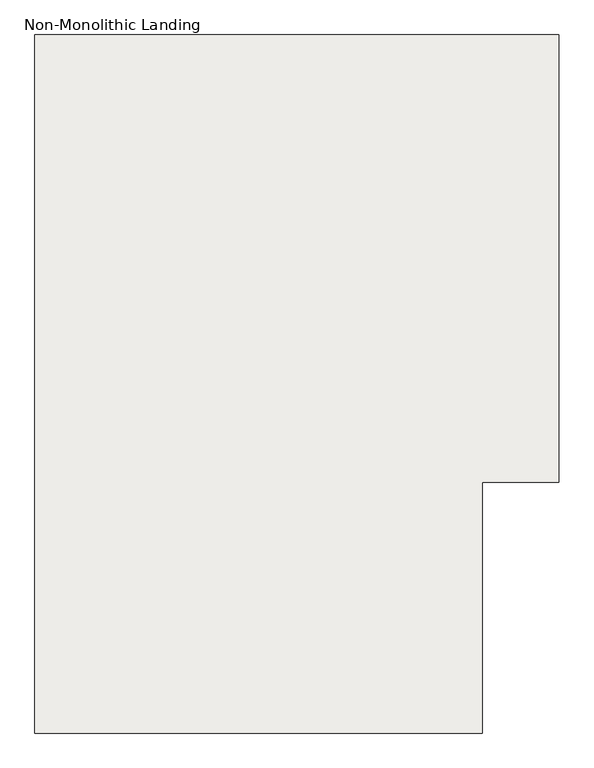
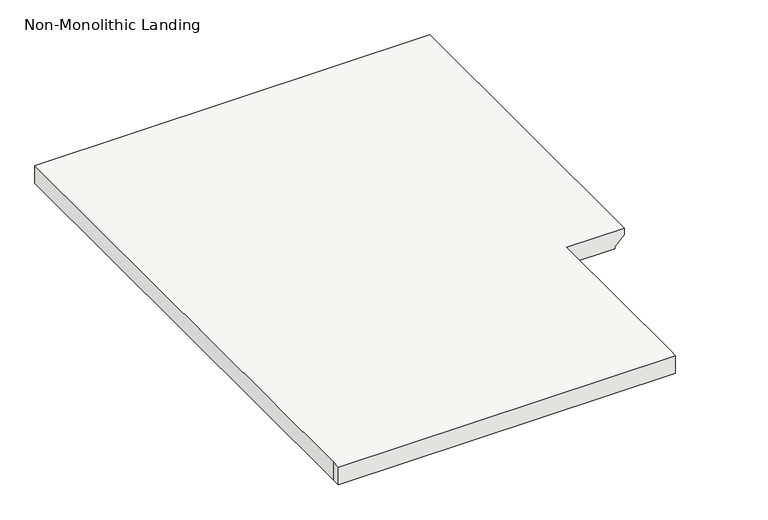
"""IFC4 building model written with IfcOpenShell, lengths in millimetres: slab geometry, Non-Monolithic Landing."""

from ifc_helpers import new_model, si_unit, origin, place, context, project, spatial, faceted_brep, source, transform, mapped, element, save


def non_monolithic_landing_bb2b3a88(model_context):
    return source(origin(), model_context, "Body", "Brep", [
        faceted_brep([(-10197.3156858, 1045.1115003, 1132.4166667), (-10197.3156858, 1045.1115003, 1151.4666667), (-10197.3156858, 130.7115003, 1151.4666667), (-10197.3156858, 130.7115003, 1132.4166667), (-10222.7156858, 1045.1115003, 1107.0166667), (-10222.7156858, 130.7115003, 1107.0166667), (-11268.1522729, 1045.1115003, 1151.4666667), (-11268.1522729, -356.3993654, 1151.4666667), (-11268.1522729, -381.7993654, 1151.4666667), (-10353.7522729, -381.7993654, 1151.4666667), (-10353.7522729, -356.3993654, 1151.4666667), (-10353.7522729, 130.7115003, 1151.4666667), (-10222.7156858, 1045.1115003, 1100.6666667), (-10222.7156858, 130.7115003, 1100.6666667), (-10353.7522729, 130.7115003, 1100.6666667), (-10353.7522729, -356.3993654, 1100.6666667), (-10353.7522729, -381.7993654, 1100.6666667), (-11268.1522729, -381.7993654, 1100.6666667), (-11268.1522729, -356.3993654, 1100.6666667), (-11268.1522729, 1045.1115003, 1100.6666667)], [[[0, 1, 2, 3]], [[4, 0, 3, 5]], [[6, 7, 8, 9, 10, 11, 2, 1]], [[12, 13, 14, 15, 16, 17, 18, 19]], [[13, 12, 4, 5]], [[6, 1, 0, 4, 12, 19]], [[7, 6, 19, 18]], [[8, 7, 18, 17]], [[9, 8, 17, 16]], [[10, 9, 16, 15]], [[11, 10, 15, 14]], [[2, 11, 14, 13, 5, 3]]]),
    ])


if __name__ == "__main__":
    model = new_model("IFC4")
    model_context = context("Model", 3, world=origin())
    ifc_project = project(units=[si_unit("LENGTHUNIT", "METRE", prefix="MILLI")], contexts=[model_context])
    site = spatial("IfcSite", under=ifc_project)
    building = spatial("IfcBuilding", under=site)
    placement = place(None, origin())
    non_monolithic_landing_shape = non_monolithic_landing_bb2b3a88(model_context)
    element("IfcSlab", 1, ObjectType="Non-Monolithic Landing", at=placement, inside=building, context=model_context, shape_type="MappedRepresentation", body=[
        mapped(non_monolithic_landing_shape, transform((0.0, 0.0, 0.0), x_axis=(1.0, 0.0, 0.0), y_axis=(0.0, 1.0, 0.0), z_axis=(0.0, 0.0, 1.0))),
    ])
    save(model, "model.ifc")
